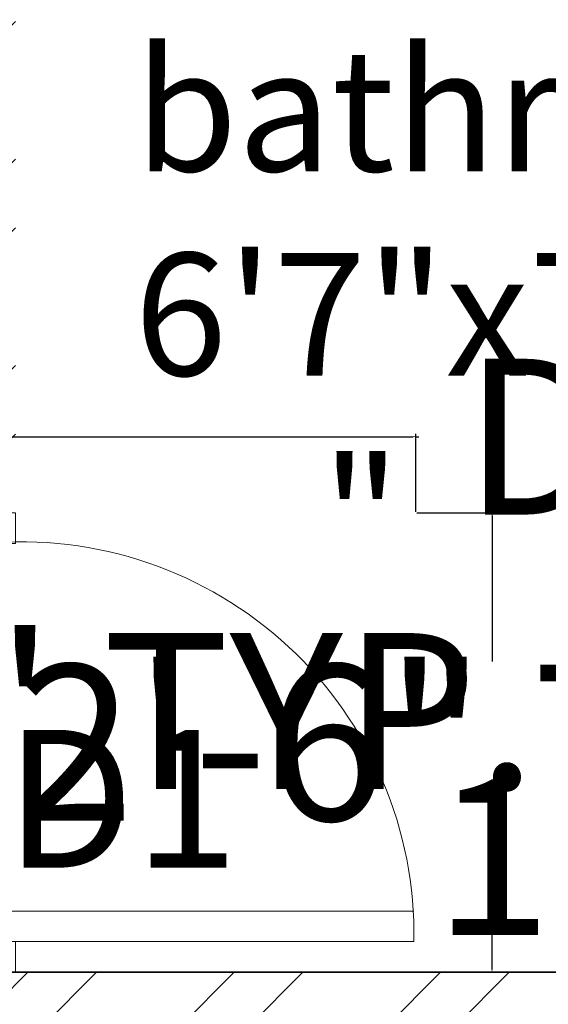
# Model space of a CAD drawing. Units: inches. Extents: x 2379 to 3013, y 1431 to 2110.
# Tile 7 of 10: x 2696 to 2730, y 1927 to 1991. Entities that reach past the tile are written whole.
import ezdxf

# ---------------------------------------------------------------- set-up
doc = ezdxf.new("R2010")
doc.units = ezdxf.units.IN
for name, color, linetype, lineweight in [('A-ANNO-DIMS', 2, 'Continuous', 18), ('A-ANNO-TEXT', 7, 'Continuous', 18), ('A-AREA-IDEN', 7, 'Continuous', 18), ('A-DOOR', 4, 'Continuous', 18), ('A-WALL-PATT', 8, 'Continuous', 13), ('A_FUR 1', 5, 'Continuous', 5), ('WALL', 7, 'Continuous', 35)]:
    doc.layers.add(name, color=color, linetype=linetype, lineweight=lineweight)
doc.styles.get("Standard").update_dxf_attribs({"font": 'arial.ttf'})
doc.dimstyles.get("Standard").update_dxf_attribs({"dimtxt": 10.18, "dimasz": 0.18, "dimexe": 0.18, "dimexo": 0.0625, "dimgap": 0.09, "dimtad": 0, "dimtih": 1, "dimtoh": 1, "dimdec": 0, "dimzin": 0, "dimdsep": 46, "dimlunit": 3, "dimtxsty": 'Standard', "dimcen": 0.09, "dimadec": 0, "dimazin": 0, "dimtfac": 1, "dimtdec": 0, "dimtofl": 0, "dimtmove": 0, "dimatfit": 3, "dimfxl": 1, "dimtolj": 1, "dimtzin": 0, "dimarcsym": 0})

# ---------------------------------------------------------------- blocks, each defined once
blk = doc.blocks.new('ESTSET')
at = {"layer": 'A_FUR 1'}
for p, q in [((-10.44359699611232, 4.096573562603225), (-10.44359699611232, 32.09657356260323)), ((-8.44359699611232, 4.096573562603225), (-8.44359699611232, 32.09657356260323)), ((-36.44359699611232, 6.096573562603225), (-36.44359699611232, 3.096573562603225)), ((-34.44359699611232, 6.096573562603225), (-36.44359699611232, 6.096573562603225)), ((-34.44359699611232, 4.096573562603225), (-34.44359699611232, 6.096573562603225)), ((-34.44359699611232, 4.096573562603225), (-34.44359699611232, 6.096573562603225)), ((-8.44359699611232, 4.096573562603225), (-8.44359699611232, 6.096573562603225)), ((-8.44359699611232, 6.096573562603225), (-6.443596996112319, 6.096573562603225)), ((-8.44359699611232, 4.096573562603225), (-8.44359699611232, 6.096573562603225)), ((-6.443596996112319, 6.096573562603225), (-6.443596996112319, 3.096573562603225)), ((-32.44359699611232, 4.096573562603225), (-34.44359699611232, 4.096573562603225)), ((-32.44359699611232, 4.096573562603225), (-34.44359699611232, 4.096573562603225)), ((-32.44359699611232, 3.096573562603225), (-32.44359699611232, 4.096573562603225)), ((-10.44359699611232, 3.096573562603225), (-10.44359699611232, 4.096573562603225)), ((-10.44359699611232, 4.096573562603225), (-8.44359699611232, 4.096573562603225)), ((-10.44359699611232, 4.096573562603225), (-8.44359699611232, 4.096573562603225)), ((-6.443596996112319, 2.096573562601521), (-36.4435969961196, 2.09657356260334)), ((-35.44359699611232, 2.096573562603225), (-33.44359699611232, 2.096573562603225)), ((-7.443596996112319, 2.096573562603225), (-9.44359699611232, 2.096573562603225))]:
    blk.add_line(p, q, dxfattribs=at)
for points in [[(-21.44359699614506, 2.09657356260334), (-18.67227073841423, 2.09657356260334), (-18.67227073841423, 5.101808480258228), (-20.05793386727964, 5.101808480258228)], [(-20.05793386727964, 5.101808480258228), (-20.05793386727964, -0.9086613550515485)], [(-21.44359699614506, 2.09657356260334), (-21.44359699614506, -0.9086613550515485), (-20.05793386727964, -0.9086613550515485)]]:
    blk.add_lwpolyline(points, dxfattribs=at)
for centre, radius, start, end in [((-8.908777800232201, 6.457098594999479), 25.64369454261379, 88.96058819788949, 185.2816045955121), ((-35.44359699611232, 3.096573562603225), 1, 180, 270), ((-33.44359699611232, 3.096573562603225), 1, 270, 0), ((-9.44359699611232, 3.096573562603225), 1, 180, 270), ((-7.443596996112319, 3.096573562603225), 1, 270, 0)]:
    blk.add_arc(centre, radius, start, end, dxfattribs=at)
blk = doc.blocks.new('*D26')
at = {"layer": 'A-ANNO-DIMS', "color": 0, "lineweight": -2, "transparency": 16777216}
for p, q in [((2688.622898699378, 1958.67097978589), (2688.622898699378, 1963.759108581785)), ((2688.802898699378, 1963.579108581785), (2721.580424005343, 1963.579108581785)), ((2721.760424005343, 1958.67097978589), (2721.760424005343, 1963.759108581785)), ((2721.760424005343, 1963.579108581785), (2721.940424005343, 1963.579108581785))]:
    blk.add_line(p, q, dxfattribs=at)
at = {"layer": 'A-ANNO-DIMS', "color": 0, "transparency": 16777216}
for points in [[(2688.802898699378, 1963.609108581785), (2688.802898699378, 1963.549108581785), (2688.622898699378, 1963.579108581785)], [(2721.580424005343, 1963.609108581785), (2721.580424005343, 1963.549108581785), (2721.760424005343, 1963.579108581785)]]:
    blk.add_solid(points, dxfattribs=at)
at = {"layer": 'Defpoints', "color": 0, "transparency": 16777216}
for p in [(2721.760424005343, 1963.579108581785), (2688.622898699378, 1958.60847978589), (2721.760424005343, 1958.60847978589)]:
    blk.add_point(p, dxfattribs=at)
at = {"layer": 'A-ANNO-DIMS', "color": 0, "transparency": 16777216, "insert": (2787.176174346408, 1963.579108581785), "char_height": 10.18, "attachment_point": 5}
blk.add_mtext('\\A1;DOOR D1 2\'-9" TYP.', dxfattribs=at)
blk = doc.blocks.new('*D27')
at = {"layer": 'A-ANNO-DIMS', "color": 0, "lineweight": -2, "transparency": 16777216}
for p, q in [((2721.822924005344, 1958.608479785891), (2726.91105280124, 1958.608479785891)), ((2726.73105280124, 1958.428479785891), (2726.73105280124, 1948.896112800894)), ((2726.73105280124, 1928.788479785884), (2726.73105280124, 1938.320846770881)), ((2721.822924005344, 1928.608479785884), (2726.91105280124, 1928.608479785884))]:
    blk.add_line(p, q, dxfattribs=at)
at = {"layer": 'A-ANNO-DIMS', "color": 0, "transparency": 16777216}
for points in [[(2726.701052801239, 1958.428479785891), (2726.76105280124, 1958.428479785891), (2726.73105280124, 1958.608479785891)], [(2726.701052801239, 1928.788479785884), (2726.76105280124, 1928.788479785884), (2726.73105280124, 1928.608479785884)]]:
    blk.add_solid(points, dxfattribs=at)
at = {"layer": 'Defpoints', "color": 0, "transparency": 16777216}
for p in [(2721.760424005344, 1958.608479785891), (2721.760424005344, 1928.608479785884), (2726.73105280124, 1928.608479785884)]:
    blk.add_point(p, dxfattribs=at)
at = {"layer": 'A-ANNO-DIMS', "color": 0, "transparency": 16777216, "insert": (2726.73105280124, 1943.608479785886), "char_height": 10.18, "attachment_point": 5}
blk.add_mtext('\\A1;2\'-6" TYP.', dxfattribs=at)
blk = doc.blocks.new('*D40')
at = {"layer": 'A-ANNO-DIMS', "color": 0, "lineweight": -2, "transparency": 16777216}
for p, q in [((2676.995321732777, 2012.608480178204), (2681.188134232791, 2012.608480178204)), ((2681.008134232791, 2012.428480178203), (2681.008134232791, 2004.381178848007)), ((2681.008134232791, 1985.619730178112), (2681.008134232791, 1993.667031508307)), ((2676.995321732777, 1985.439730178112), (2681.188134232791, 1985.439730178112))]:
    blk.add_line(p, q, dxfattribs=at)
at = {"layer": 'A-ANNO-DIMS', "color": 0, "transparency": 16777216}
for points in [[(2680.978134232791, 2012.428480178203), (2681.038134232792, 2012.428480178203), (2681.008134232791, 2012.608480178204)], [(2680.978134232791, 1985.619730178112), (2681.038134232792, 1985.619730178112), (2681.008134232791, 1985.439730178112)]]:
    blk.add_solid(points, dxfattribs=at)
at = {"layer": 'Defpoints', "color": 0, "transparency": 16777216}
for p in [(2676.932821732777, 2012.608480178204), (2681.008134232791, 2012.608480178204), (2676.932821732777, 1985.439730178112)]:
    blk.add_point(p, dxfattribs=at)
at = {"layer": 'A-ANNO-DIMS', "color": 0, "transparency": 16777216, "insert": (2681.008134232791, 1999.024105178156), "char_height": 10.18, "attachment_point": 5}
blk.add_mtext('\\A1;WC 2\'-3" TYP.', dxfattribs=at)
blk = doc.blocks.new('*D42')
at = {"layer": 'A-ANNO-DIMS', "color": 0, "lineweight": -2, "transparency": 16777216}
for p, q in [((2731.292496124008, 1945.667853308336), (2731.112496124008, 1945.667853308336)), ((2731.292496124008, 1942.76850560317), (2731.292496124008, 1945.847853308336)), ((2750.858147491776, 1945.667853308336), (2731.472496124008, 1945.667853308336)), ((2751.038147491776, 1942.76850560317), (2751.038147491776, 1945.847853308336))]:
    blk.add_line(p, q, dxfattribs=at)
at = {"layer": 'A-ANNO-DIMS', "color": 0, "transparency": 16777216}
for points in [[(2731.472496124008, 1945.697853308336), (2731.472496124008, 1945.637853308335), (2731.292496124008, 1945.667853308336)], [(2750.858147491776, 1945.697853308336), (2750.858147491776, 1945.637853308335), (2751.038147491776, 1945.667853308336)]]:
    blk.add_solid(points, dxfattribs=at)
at = {"layer": 'Defpoints', "color": 0, "transparency": 16777216}
for p in [(2731.292496124008, 1945.667853308336), (2731.292496124008, 1942.70600560317), (2751.038147491776, 1942.70600560317)]:
    blk.add_point(p, dxfattribs=at)
at = {"layer": 'A-ANNO-DIMS', "color": 0, "transparency": 16777216, "insert": (2665.046929957569, 1945.667853308336), "char_height": 10.18, "attachment_point": 5}
blk.add_mtext('\\A1;BASIN 1\'-7 1/2" TYP.', dxfattribs=at)
blk = doc.blocks.new('*D43')
at = {"layer": 'A-ANNO-DIMS', "color": 0, "lineweight": -2, "transparency": 16777216}
for p, q in [((2751.100647491777, 1942.706005603171), (2754.179995196943, 1942.706005603171)), ((2753.999995196943, 1942.526005603171), (2753.999995196943, 1941.328426043108)), ((2753.999995196943, 1929.722238024655), (2753.999995196943, 1930.919817584718)), ((2751.100647491777, 1929.542238024655), (2754.179995196943, 1929.542238024655))]:
    blk.add_line(p, q, dxfattribs=at)
at = {"layer": 'A-ANNO-DIMS', "color": 0, "transparency": 16777216}
for points in [[(2753.969995196943, 1942.526005603171), (2754.029995196944, 1942.526005603171), (2753.999995196943, 1942.706005603171)], [(2753.969995196943, 1929.722238024655), (2754.029995196944, 1929.722238024655), (2753.999995196943, 1929.542238024655)]]:
    blk.add_solid(points, dxfattribs=at)
at = {"layer": 'Defpoints', "color": 0, "transparency": 16777216}
for p in [(2751.038147491777, 1942.706005603171), (2753.999995196943, 1942.706005603171), (2751.038147491777, 1929.542238024655)]:
    blk.add_point(p, dxfattribs=at)
at = {"layer": 'A-ANNO-DIMS', "color": 0, "transparency": 16777216, "insert": (2753.999995196943, 1936.124121813912), "char_height": 10.18, "attachment_point": 5}
blk.add_mtext('\\A1;1\'-1" TYP.', dxfattribs=at)
blk = doc.blocks.new('*D46')
at = {"layer": 'A-ANNO-DIMS', "color": 0, "lineweight": -2, "transparency": 16777216}
for p, q in [((2736.087387447885, 2012.608480178147), (2737.933387607347, 2012.608480178147)), ((2737.753387607348, 2012.428480178146), (2737.753387607348, 2012.203886649792)), ((2737.753387607348, 2001.265145781737), (2737.753387607348, 2001.489739310092)), ((2736.087387447885, 2001.085145781737), (2737.933387607347, 2001.085145781737))]:
    blk.add_line(p, q, dxfattribs=at)
at = {"layer": 'A-ANNO-DIMS', "color": 0, "transparency": 16777216}
for points in [[(2737.723387607348, 2012.428480178146), (2737.783387607348, 2012.428480178146), (2737.753387607348, 2012.608480178147)], [(2737.723387607348, 2001.265145781737), (2737.783387607348, 2001.265145781737), (2737.753387607348, 2001.085145781737)]]:
    blk.add_solid(points, dxfattribs=at)
at = {"layer": 'Defpoints', "color": 0, "transparency": 16777216}
for p in [(2736.024887447885, 2012.608480178147), (2737.753387607348, 2012.608480178147), (2736.024887447885, 2001.085145781737)]:
    blk.add_point(p, dxfattribs=at)
at = {"layer": 'A-ANNO-DIMS', "color": 0, "transparency": 16777216, "insert": (2737.753387607348, 2006.84681297994), "char_height": 10.18, "attachment_point": 5}
blk.add_mtext('\\A1;SHOWER 0\'-11 1/2"', dxfattribs=at)

msp = doc.modelspace()

# ---------------------------------------------------------------- hatches: boundary and pattern name
at = {"layer": 'A-WALL-PATT'}
h = msp.add_hatch(dxfattribs=at)
h.set_pattern_fill('ANSI32', color=256)
h.set_pattern_definition([(45, (0, 0), (-6.735192090801865, 6.735192090801866), []), (45, (4.49013, 0), (-6.735192090801865, 6.735192090801866), [])])
h.paths.add_polyline_path([(2925.628133617025, 1862.608480178145), (2815.628133617027, 1862.608480178145), (2815.628133617026, 1858.608480178145), (2827.628133617026, 1858.608480178145), (2827.62813361702, 1810.608480178145), (2815.628133617021, 1810.608480178145), (2815.62813361702, 1806.608480178145), (2850.776028957045, 1806.608480178145), (2850.776028957045, 1810.608480178145), (2831.628133617021, 1810.608480178145), (2831.628133617026, 1858.608480178145), (2925.628133617025, 1858.608480178145)])
h.paths.add_polyline_path([(2925.628133617025, 1810.608480178145), (2880.776028957045, 1810.608480178145), (2880.776028957046, 1806.608480178145), (2925.628133617025, 1806.608480178145)], flags=17)
h.paths.add_polyline_path([(2633.752023401108, 1660.608480178145), (2594.628133617026, 1660.608480178145), (2481.628132350232, 1660.608480178145), (2481.628132350232, 1651.608480178145), (2588.628133617025, 1651.608480178145), (2588.628133617025, 1570.608480178146), (2624.284264477168, 1570.608480178146), (2624.284264477168, 1574.608480178146), (2592.628133617025, 1574.608480178146), (2592.628133617025, 1651.608480178145), (2633.752023401108, 1651.608480178145)])
h.paths.add_polyline_path([(2594.628133617025, 1809.608480178145), (2481.628132350232, 1809.608480178145), (2481.628132350232, 1805.608480178145), (2594.628133617025, 1805.608480178145)])
h.paths.add_polyline_path([(2594.628133617025, 2012.608480178145), (2597.21307907444, 2012.608480178145), (2597.21307907444, 2021.608480178145), (2588.21307907444, 2021.608480178145), (2588.21307907444, 2012.608480178145), (2590.628133617026, 2012.608480178145), (2590.628133617025, 1845.608480178145), (2594.628133617025, 1845.608480178145)])
h.paths.add_polyline_path([(2767.628133617026, 2012.608480178145), (2770.26658329333, 2012.608480178145), (2770.26658329333, 2021.608480178145), (2761.26658329333, 2021.608480178145), (2761.26658329333, 2012.608480178145), (2763.628133617026, 2012.608480178145), (2763.628133617026, 1928.608480178145), (2691.628133617026, 1928.608480178146), (2643.628133617026, 1928.608480178146), (2643.628133617026, 1924.608480178146), (2691.628133617026, 1924.608480178145), (2763.628133617026, 1924.608480178145), (2763.628133617026, 1858.608480178145), (2779.628133617026, 1858.608480178145), (2779.628133617026, 1862.608480178145), (2767.628133617026, 1862.608480178145)])
h.paths.add_polyline_path([(2613.628133617026, 2012.608480178146), (2613.628133617026, 2021.608480178145), (2597.21307907444, 2021.608480178145), (2597.21307907444, 2012.608480178145)])
h.paths.add_polyline_path([(2508.325157742558, 2012.608480178146), (2508.325157742557, 2021.608480178145), (2478.628133617025, 2021.608480178145), (2478.628133617025, 2012.608480178145)])
h.paths.add_polyline_path([(2556.325157742558, 2021.608480178145), (2556.325157742558, 2012.608480178145), (2588.21307907444, 2012.608480178145), (2588.21307907444, 2021.608480178145)])
h.paths.add_polyline_path([(2659.149603475649, 2012.608480178146), (2659.149603475649, 2021.608480178145), (2643.628133617026, 2021.608480178145), (2643.628133617025, 1958.608480178146), (2661.628133617025, 1958.608480178146), (2661.628133617026, 1962.608480178146), (2647.628133617026, 1962.608480178146), (2647.628133617026, 2012.608480178145)])
h.paths.add_polyline_path([(2714.172783852811, 2012.608480178145), (2714.172783852811, 2021.608480178145), (2683.149603475648, 2021.608480178145), (2683.149603475648, 2012.608480178145), (2691.628133617026, 2012.608480178145), (2691.628133617026, 1958.608480178146), (2695.628133617026, 1958.608480178146), (2695.628133617026, 2012.608480178145)])
h.paths.add_polyline_path([(2738.172783852812, 2021.608480178145), (2738.172783852811, 2012.608480178145), (2761.26658329333, 2012.608480178145), (2761.26658329333, 2021.608480178145)])
h.paths.add_polyline_path([(2820.757909975796, 2012.608480178145), (2820.757909975796, 2021.608480178145), (2770.26658329333, 2021.608480178145), (2770.26658329333, 2012.608480178145)])
h.paths.add_polyline_path([(2868.757909975796, 2021.608480178145), (2868.757909975795, 2012.608480178145), (2928.628133542687, 2012.608480178145), (2928.628133542687, 2021.608480178145)])
h.paths.add_polyline_path([(2928.628133617026, 1962.897453102627), (2937.628133617025, 1962.897453102627), (2937.628133617025, 2009.608480178145), (2928.628133617026, 2009.608480178145)])
h.paths.add_polyline_path([(2937.628133617025, 1914.897453102627), (2928.628133617026, 1914.897453102627), (2928.628133617026, 1863.796245476747), (2937.628133617025, 1863.796245476747)])
h.paths.add_polyline_path([(2928.628133617025, 1846.587382132453), (2937.628133617025, 1846.587382132453), (2937.628133617025, 1854.796245476746), (2928.628133617026, 1854.796245476746)])
h.paths.add_polyline_path([(2937.628133617025, 1822.587382132453), (2928.628133617025, 1822.587382132453), (2928.628133617025, 1813.620125754823), (2937.628133617025, 1813.620125754823)])
h.paths.add_polyline_path([(2928.628133617025, 1778.475127785104), (2937.628133617026, 1778.475127785104), (2937.628133617025, 1813.620125754823), (2928.628133617025, 1813.620125754823), (2928.628133617025, 1810.608480178145), (2925.628133617025, 1810.608480178145), (2925.628133617025, 1806.608480178145), (2928.628133617025, 1806.608480178145)])
h.paths.add_polyline_path([(2816.219214803751, 1651.608480178145), (2816.219214803751, 1660.608480178145), (2767.628133617025, 1660.608480178145), (2767.628133617025, 1806.608480178145), (2779.62813361702, 1806.608480178145), (2779.62813361702, 1810.608480178145), (2763.628133617026, 1810.608480178145), (2763.628133617025, 1660.608480178145), (2688.628133617025, 1660.608480178145), (2688.628133617026, 1810.608480178144), (2684.628133617026, 1810.608480178145), (2684.628133617025, 1660.608480178145), (2669.752023401108, 1660.608480178145), (2669.752023401108, 1651.608480178145), (2763.628133617025, 1651.608480178145), (2763.628133617025, 1574.608480178145), (2672.284264477169, 1574.608480178145), (2672.284264477168, 1570.608480178145), (2767.628133617026, 1570.608480178145), (2767.628133617026, 1651.608480178145)])
h.paths.add_polyline_path([(2864.219214803751, 1660.608480178145), (2864.219214803751, 1651.608480178145), (2937.628133617025, 1651.608480178145), (2937.628133617026, 1730.475127785104), (2928.628133617025, 1730.475127785104), (2928.628133617025, 1660.608480178145)])
h.paths.add_polyline_path([(2469.628133617026, 1975.187574086886), (2478.628133617025, 1975.187574086886), (2478.628133617025, 2009.608480178146), (2469.628133617025, 2009.608480178146)])
h.paths.add_polyline_path([(2478.628133617025, 1927.187574086886), (2469.628133617026, 1927.187574086886), (2469.628133617025, 1811.017018303813), (2478.628133617025, 1811.017018303813)])
h.paths.add_polyline_path([(2469.628133617025, 1758.038369990633), (2478.628133617025, 1758.038369990633), (2478.628133617025, 1802.017018303813), (2469.628133617025, 1802.017018303813)])
h.paths.add_polyline_path([(2478.628133617025, 1710.038369990633), (2469.628133617025, 1710.038369990633), (2469.628133617025, 1660.608479805985), (2478.628133617025, 1660.608479805985)])

# ---------------------------------------------------------------- linework, layer by layer
at = {"layer": 'WALL'}
msp.add_line((2691.628133617026, 1928.608480178146), (2763.628133617025, 1928.608480178145), dxfattribs=at)

# ---------------------------------------------------------------- block references
at = {"layer": 'A-DOOR', "rotation": 270}
msp.add_blockref('ESTSET', (2689.53156005443, 1922.164882789771), dxfattribs=at)

# ---------------------------------------------------------------- texts
at = {"layer": 'A-ANNO-TEXT', "insert": (2694.91956702049, 1944.43683036302), "char_height": 9, "attachment_point": 1}
msp.add_mtext_dynamic_manual_height_columns('D1', width=106.8918998292883, gutter_width=12.5, heights=[0], dxfattribs=at)
at = {"layer": 'A-AREA-IDEN', "insert": (2703.367587553309, 1988.906750283259), "char_height": 8, "attachment_point": 1}
msp.add_mtext_dynamic_manual_height_columns('bathroom\\P6\'7"x7\'          "  ', width=46.15057788734339, gutter_width=12.5, heights=[0], dxfattribs=at)

# ---------------------------------------------------------------- dimensions: what is measured, and where the dimension line sits
at = {"layer": 'A-ANNO-DIMS'}
for base, p1, p2, angle, text, picture, middle in [((2737.753387607348, 2012.608480178147), (2736.024887447884, 2001.085145781736), (2736.024887447884, 2012.608480178146), 90, 'SHOWER <>', '*D46', (2737.753387607348, 2006.84681297994)), ((2681.008134232791, 2012.608480178204), (2676.932821732776, 1985.439730178111), (2676.932821732776, 2012.608480178203), 90, 'WC <> TYP.', '*D40', (2681.008134232791, 1999.024105178156)), ((2731.292496124008, 1945.667853308336), (2751.038147491776, 1942.70600560317), (2731.292496124008, 1942.70600560317), 180, 'BASIN <> TYP.', '*D42', (2665.046929957569, 1945.667853308336)), ((2726.73105280124, 1928.608479785884), (2721.760424005343, 1958.60847978589), (2721.760424005343, 1928.608479785883), 270, '<> TYP.', '*D27', (2726.73105280124, 1943.608479785886)), ((2753.999995196943, 1942.706005603171), (2751.038147491776, 1929.542238024654), (2751.038147491776, 1942.70600560317), 90, '<> TYP.', '*D43', (2753.999995196943, 1936.124121813912))]:
    dim = msp.add_linear_dim(base=base, p1=p1, p2=p2, angle=angle, text=text, dimstyle='Standard', override={"dimdec": 1, "dimlfac": 1, "dimrnd": 0, "dimzin": 1, "dimdsep": 46, "dimlunit": 4, "dimfrac": 2}, dxfattribs=at)
    dim.commit()
    dim.dimension.update_dxf_attribs({"geometry": picture, "text_midpoint": middle})
dim = msp.add_linear_dim(base=(2721.760424005343, 1963.579108581785), p1=(2688.622898699378, 1958.60847978589), p2=(2721.760424005343, 1958.60847978589), text='DOOR D1 <> TYP.', dimstyle='Standard', override={"dimdec": 1, "dimlfac": 1, "dimrnd": 0, "dimzin": 1, "dimdsep": 46, "dimlunit": 4, "dimfrac": 2}, dxfattribs=at)
dim.commit()
dim.dimension.update_dxf_attribs({"geometry": '*D26', "text_midpoint": (2787.176174346408, 1963.579108581785)})

doc.saveas('drawing.dxf')
